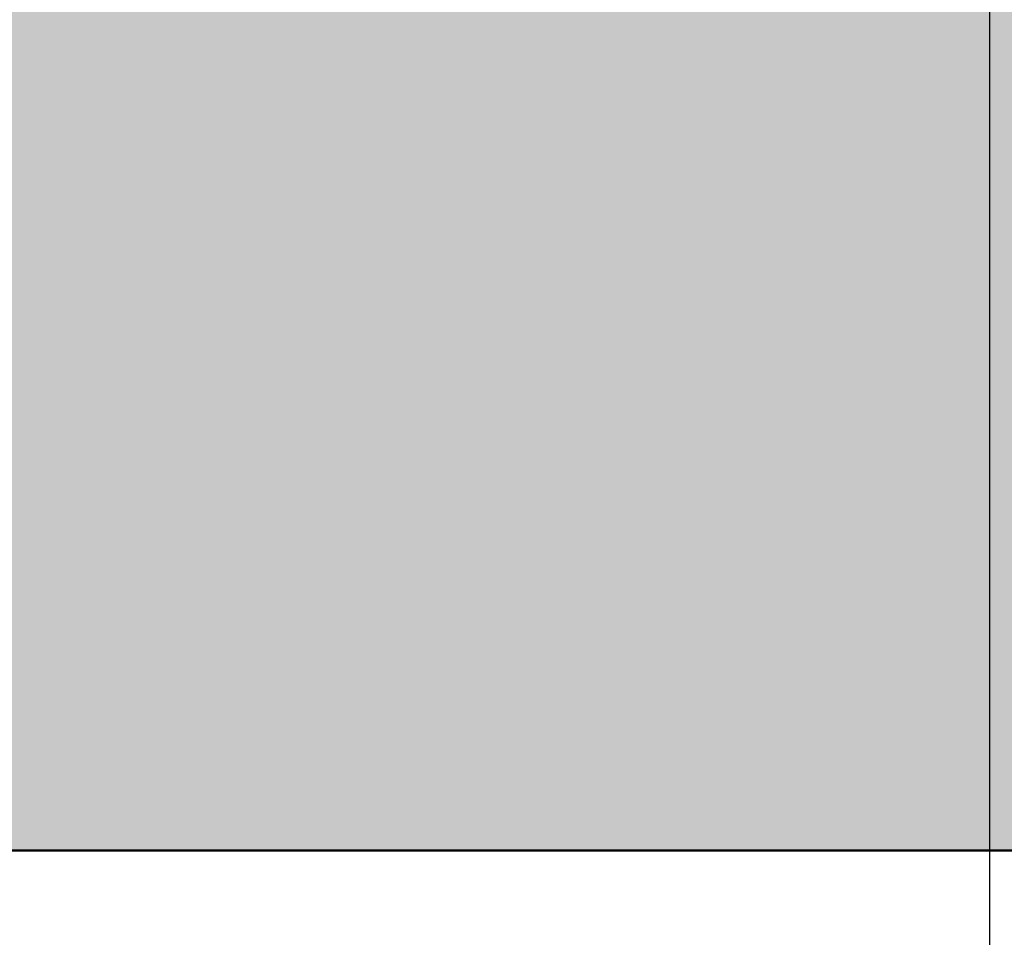
# Model space of a CAD drawing. Units: millimetres. Extents: x 0 to 2267, y 0 to 1823.
# Tile 140 of 256: x 1802 to 1844, y 1074 to 1113. Entities that reach past the tile are written whole.
import ezdxf

# ---------------------------------------------------------------- set-up
doc = ezdxf.new("R2010")
doc.units = ezdxf.units.MM
doc.header["$MEASUREMENT"] = 0
for name, color, linetype, lineweight in [('M-DIMS', 2, 'Continuous', 25), ('M-HATC', 252, 'Continuous', 18), ('M-OUTL', 7, 'Continuous', 50)]:
    doc.layers.add(name, color=color, linetype=linetype, lineweight=lineweight)
doc.styles.get("Standard").update_dxf_attribs({"font": 'arial.ttf'})
doc.dimstyles.get("Standard").update_dxf_attribs({"dimtxt": 7, "dimasz": 4, "dimexe": 0.18, "dimexo": 0.0625, "dimgap": 0.09, "dimtad": 0, "dimdec": 0, "dimzin": 0, "dimdsep": 46, "dimtxsty": 'Standard', "dimcen": 0.09, "dimadec": 0, "dimazin": 0, "dimtfac": 1, "dimtdec": 0, "dimtofl": 0, "dimtmove": 0, "dimatfit": 3, "dimfxl": 1, "dimtolj": 1, "dimtzin": 0, "dimarcsym": 0})

# ---------------------------------------------------------------- blocks, each defined once
blk = doc.blocks.new('*D1')
at = {"layer": 'Defpoints', "color": 0, "transparency": 16777216}
for p in [(1593.429, 1127.417), (1843.429, 1127.417), (1843.429, 955.628)]:
    blk.add_point(p, dxfattribs=at)
at = {"layer": 'M-DIMS', "color": 0, "lineweight": -2, "transparency": 16777216}
for p, q in [((1593.429, 1127.355), (1593.429, 955.448)), ((1843.429, 1127.355), (1843.429, 955.448)), ((1597.429, 955.628), (1710.558, 955.628)), ((1839.429, 955.628), (1726.3, 955.628))]:
    blk.add_line(p, q, dxfattribs=at)
at = {"layer": 'M-DIMS', "color": 0, "transparency": 16777216}
for points in [[(1597.429, 956.294), (1597.429, 954.961), (1593.429, 955.628)], [(1839.429, 956.294), (1839.429, 954.961), (1843.429, 955.628)]]:
    blk.add_solid(points, dxfattribs=at)
at = {"layer": 'M-DIMS', "color": 0, "transparency": 16777216, "insert": (1718.429, 955.628), "char_height": 7, "attachment_point": 5}
blk.add_mtext('\\A1;250', dxfattribs=at)
blk = doc.blocks.new('*D2')
at = {"layer": 'Defpoints', "color": 0, "transparency": 16777216}
for p in [(1505.929, 1077.417), (1930.929, 1077.417), (1930.929, 906.787)]:
    blk.add_point(p, dxfattribs=at)
at = {"layer": 'M-DIMS', "color": 0, "lineweight": -2, "transparency": 16777216}
for p, q in [((1505.929, 1077.355), (1505.929, 906.607)), ((1930.929, 1077.355), (1930.929, 906.607)), ((1509.929, 906.787), (1710.439, 906.787)), ((1926.929, 906.787), (1726.419, 906.787))]:
    blk.add_line(p, q, dxfattribs=at)
at = {"layer": 'M-DIMS', "color": 0, "transparency": 16777216}
for points in [[(1509.929, 907.453), (1509.929, 906.12), (1505.929, 906.787)], [(1926.929, 907.453), (1926.929, 906.12), (1930.929, 906.787)]]:
    blk.add_solid(points, dxfattribs=at)
at = {"layer": 'M-DIMS', "color": 0, "transparency": 16777216, "insert": (1718.429, 906.787), "char_height": 7, "attachment_point": 5}
blk.add_mtext('\\A1;425', dxfattribs=at)

msp = doc.modelspace()

# ---------------------------------------------------------------- hatches: boundary and pattern name
at = {"layer": 'M-HATC'}
h = msp.add_hatch(color=256, dxfattribs=at)
h.dxf.hatch_style = 1
h.paths.add_polyline_path([(2065.771, 1618.062, 0.236068), (2055.771, 1638.062), (1381.087, 1638.062, 0.236068), (1371.087, 1618.062), (1371.087, 1603.062), (2055.771, 1603.062), (2065.771, 1603.062)])
h.paths.add_polyline_path([(2062.772, 1550.296), (2062.772, 1560.296), (1374.086, 1560.296), (1374.086, 1550.296), (1374.086, 1540.296), (1384.086, 1540.296), (1389.086, 1540.296), (2062.772, 1540.296)])
h.paths.add_polyline_path([(1930.929, 1282.766), (1505.929, 1282.766), (1587.628, 1235.597, 0.131652), (1600.128, 1232.247), (1836.73, 1232.247, 0.131652), (1849.23, 1235.597)])
h.paths.add_polyline_path([(1930.929, 1117.417), (1905.929, 1117.417), (1505.929, 1117.417), (1505.929, 1077.417), (1930.929, 1077.417)])

# ---------------------------------------------------------------- linework, layer by layer
at = {"layer": 'M-OUTL'}
msp.add_line((1505.929, 1077.417), (1930.929, 1077.417), dxfattribs=at)

# ---------------------------------------------------------------- dimensions: what is measured, and where the dimension line sits
at = {"layer": 'M-DIMS'}
for base, p1, p2, picture, middle in [((1843.429, 955.628), (1593.429, 1127.417), (1843.429, 1127.417), '*D1', (1718.429, 955.628)), ((1930.929, 906.787), (1505.929, 1077.417), (1930.929, 1077.417), '*D2', (1718.429, 906.787))]:
    dim = msp.add_linear_dim(base=base, p1=p1, p2=p2, dimstyle='Standard', override={"dimclrd": 0, "dimclre": 0, "dimclrt": 0}, dxfattribs=at)
    dim.commit()
    dim.dimension.update_dxf_attribs({"geometry": picture, "text_midpoint": middle})

doc.saveas('drawing.dxf')
